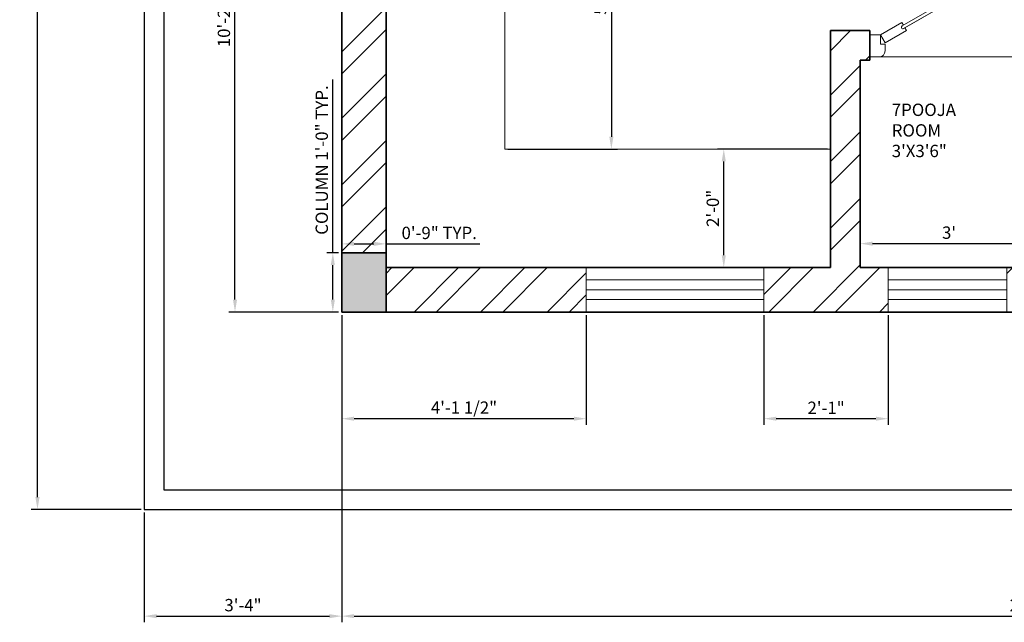
# Model space of a CAD drawing. Units: inches. Extents: x -138 to 270, y 8284 to 8764.
# Tile 1 of 10: x -138 to 61, y 8284 to 8406. Entities that reach past the tile are written whole.
import ezdxf

# ---------------------------------------------------------------- set-up
doc = ezdxf.new("R2010")
doc.units = ezdxf.units.IN
for name, color, linetype, lineweight in [('A-ANNO-DIMS', 2, 'Continuous', 18), ('A-AREA-IDEN', 7, 'Continuous', 18), ('A-FLOR-CASE', 9, 'Continuous', 18), ('C-PROP', 7, 'Continuous', 25), ('DOOR', 32, 'Continuous', 15), ('WALL', 8, 'Continuous', 35), ('WINDOW', 151, 'Continuous', 15)]:
    doc.layers.add(name, color=color, linetype=linetype, lineweight=lineweight)
doc.layers.add('A-COLS', color=252, linetype='Continuous', lineweight=35, true_color=0x939598)
doc.layers.add('A-WALL-PATT', color=32, linetype='Continuous', lineweight=9, true_color=0xbc761a)
doc.styles.get("Standard").update_dxf_attribs({"font": 'arial.ttf'})
doc.dimstyles.new('ISO-25', dxfattribs={"dimtxt": 2.5, "dimasz": 2.5, "dimexe": 1.25, "dimexo": 0.625, "dimtad": 1, "dimdec": 0, "dimlunit": 3, "dimtxsty": 'Standard', "dimcen": 2.5, "dimadec": 0, "dimazin": 0, "dimtfac": 1, "dimtdec": 0, "dimtmove": 0, "dimatfit": 3, "dimfxl": 1, "dimarcsym": 0})

# ---------------------------------------------------------------- blocks, each defined once
blk = doc.blocks.new('A$C1A8229D7')
at = {"layer": 'DOOR'}
for p, q in [((22.38, 16.16), (26.71, 18.66)), ((24.39, 17.68), (25.47, 18.3)), ((24.56, 18), (25.1, 18.31)), ((24.56, 18), (24.66, 17.83)), ((24.56, 18), (24.56, 18)), ((24.83, 18.15), (24.83, 18.15)), ((25.1, 18.31), (25.2, 18.15)), ((25.47, 18.3), (25.62, 18.03)), ((27.64, 17.03), (26.71, 18.66)), ((22.69, 15.61), (22.38, 16.16)), ((23.31, 14.53), (27.64, 17.03)), ((24.39, 17.68), (24.54, 17.41)), ((25.64, 15.51), (26.72, 16.14)), ((26.54, 15.82), (26.45, 15.98)), ((26.72, 16.14), (26.56, 16.41)), ((6.56, 6.3), (22.96, 15.77)), ((23.27, 15.23), (6.87, 5.76)), ((7.14, 5.92), (23, 15.07)), ((23.31, 14.53), (23, 15.07)), ((23.39, 15.66), (23.39, 15.66)), ((25.64, 15.51), (25.48, 15.78)), ((26, 15.51), (25.91, 15.67)), ((26, 15.51), (26.54, 15.82)), ((26, 15.51), (26, 15.51)), ((26.27, 15.66), (26.27, 15.66)), ((6.52, 7), (2.19, 4.5)), ((6.83, 6.46), (6.52, 7)), ((0, 0), (0, 4.5)), ((0, 4.5), (2.19, 4.5)), ((2.19, 2.62), (2.19, 4.5)), ((3.12, 2.88), (2.19, 4.5)), ((7.46, 5.38), (3.12, 2.88)), ((6.45, 5.88), (6.45, 5.88)), ((7.46, 5.38), (7.14, 5.92)), ((30.5, 2.62), (30.5, 4.5)), ((33, 4.5), (30.5, 4.5)), ((33, 0), (33, 4.5)), ((2.19, 2.62), (3.12, 2.62)), ((3.12, 1.25), (3.12, 2.62)), ((29.87, 1.25), (29.87, 2.62)), ((30.5, 2.62), (29.87, 2.62)), ((0, 0), (1.87, 0)), ((33, 0), (0, 0)), ((0, 0), (33, 0)), ((33, 0), (31.12, 0))]:
    blk.add_line(p, q, dxfattribs=at)
at = {"layer": 'DOOR', "ltscale": 0.1}
blk.add_arc((6.98, 5.45), 23.69, 353.1504, 56.0415, dxfattribs=at)
at = {"layer": 'DOOR'}
for centre, radius, start, end in [((25.46, 15.13), 3.63, 111.4546, 145.7774), ((27.78, 10.32), 8.61, 114.2033, 127.709), ((24.4, 17.99), 0.592, 22.7059, 117.5689), ((24.41, 17.91), 0.312, 30, 120), ((22.48, 17.15), 0.0372, 138.2373, 332.5518), ((23.12, 15.5), 0.312, 30, 120), ((23.12, 15.5), 0.312, 300, 30), ((24.23, 14.13), 0.0372, 87.4482, 281.7627), ((20.96, 22.13), 8.61, 292.291, 305.7967), ((23.97, 17.71), 3.63, 274.2226, 308.5454), ((25.85, 15.42), 0.312, 300, 30), ((25.92, 15.37), 0.592, 302.4311, 37.2941), ((6.72, 6.03), 0.312, 120, 210), ((6.72, 6.03), 0.312, 210, 300), ((1.87, 1.25), 1.25, 270, 0), ((31.12, 1.25), 1.25, 180, 270)]:
    blk.add_arc(centre, radius, start, end, dxfattribs=at)
blk = doc.blocks.new('*D24')
at = {"layer": 'A-ANNO-DIMS', "color": 0, "lineweight": -2, "transparency": 16777216}
for p, q in [((32.08, 8356.87), (32.08, 8362.34)), ((68.08, 8356.87), (68.08, 8362.34)), ((34.58, 8361.09), (65.58, 8361.09))]:
    blk.add_line(p, q, dxfattribs=at)
at = {"layer": 'A-ANNO-DIMS', "color": 0, "transparency": 16777216}
for points in [[(34.58, 8361.51), (34.58, 8360.67), (32.08, 8361.09)], [(65.58, 8361.51), (65.58, 8360.67), (68.08, 8361.09)]]:
    blk.add_solid(points, dxfattribs=at)
at = {"layer": 'Defpoints', "color": 0, "transparency": 16777216}
for p in [(68.08, 8361.09), (32.08, 8356.24), (68.08, 8356.24)]:
    blk.add_point(p, dxfattribs=at)
at = {"layer": 'A-ANNO-DIMS', "color": 0, "transparency": 16777216, "insert": (50.08, 8362.99), "char_height": 2.5, "attachment_point": 5}
blk.add_mtext("3'", dxfattribs=at)
blk = doc.blocks.new('WINDOW-36IN')
for p, q in [((0, 6.5), (36, 6.5)), ((0, 4.5), (36, 4.5)), ((0, 2.5), (36, 2.5))]:
    blk.add_line(p, q)
blk.add_lwpolyline([(0, 0), (36, 0), (36, 9), (0, 9)], close=True)
blk = doc.blocks.new('WINDOW-24IN')
for p, q in [((0, 6.5), (24, 6.5)), ((0, 4.5), (24, 4.5)), ((0, 2.5), (24, 2.5))]:
    blk.add_line(p, q)
blk.add_lwpolyline([(0, 0), (24, 0), (24, 9), (0, 9)], close=True)
blk = doc.blocks.new('COLUMN-9X12IN')
h = blk.add_hatch(color=256)
h.dxf.hatch_style = 1
h.paths.add_polyline_path([(9, 12), (0, 12), (0, 0), (9, 0)])
blk.add_lwpolyline([(0, 0), (9, 0), (9, 12), (0, 12)], close=True)
blk = doc.blocks.new('*D29')
at = {"layer": 'A-ANNO-DIMS', "color": 0, "lineweight": -2, "transparency": 16777216}
for p, q in [((-74.72, 8359.24), (-74.72, 8394.31)), ((-73.55, 8359.24), (-75.97, 8359.24)), ((-74.72, 8349.74), (-74.72, 8356.74)), ((-73.55, 8347.24), (-75.97, 8347.24))]:
    blk.add_line(p, q, dxfattribs=at)
at = {"layer": 'A-ANNO-DIMS', "color": 0, "transparency": 16777216}
for points in [[(-75.14, 8356.74), (-74.31, 8356.74), (-74.72, 8359.24)], [(-75.14, 8349.74), (-74.31, 8349.74), (-74.72, 8347.24)]]:
    blk.add_solid(points, dxfattribs=at)
at = {"layer": 'Defpoints', "color": 0, "transparency": 16777216}
for p in [(-74.72, 8359.24), (-72.92, 8359.24), (-72.92, 8347.24)]:
    blk.add_point(p, dxfattribs=at)
at = {"layer": 'A-ANNO-DIMS', "color": 0, "transparency": 16777216, "insert": (-76.64, 8378.02), "char_height": 2.5, "attachment_point": 5, "rotation": 90}
blk.add_mtext('COLUMN 1\'-0" TYP.', dxfattribs=at)
blk = doc.blocks.new('*D30')
at = {"layer": 'A-ANNO-DIMS', "color": 0, "lineweight": -2, "transparency": 16777216}
for p, q in [((-72.92, 8359.87), (-72.92, 8362.29)), ((-63.92, 8359.87), (-63.92, 8362.29)), ((-70.42, 8361.04), (-66.42, 8361.04)), ((-63.92, 8361.04), (-44.94, 8361.04))]:
    blk.add_line(p, q, dxfattribs=at)
at = {"layer": 'A-ANNO-DIMS', "color": 0, "transparency": 16777216}
for points in [[(-70.42, 8361.46), (-70.42, 8360.63), (-72.92, 8361.04)], [(-66.42, 8361.46), (-66.42, 8360.63), (-63.92, 8361.04)]]:
    blk.add_solid(points, dxfattribs=at)
at = {"layer": 'Defpoints', "color": 0, "transparency": 16777216}
for p in [(-63.92, 8361.04), (-72.92, 8359.24), (-63.92, 8359.24)]:
    blk.add_point(p, dxfattribs=at)
at = {"layer": 'A-ANNO-DIMS', "color": 0, "transparency": 16777216, "insert": (-53.18, 8362.94), "char_height": 2.5, "attachment_point": 5}
blk.add_mtext('0\'-9" TYP.', dxfattribs=at)
blk = doc.blocks.new('*D52')
at = {"layer": 'A-ANNO-DIMS', "color": 0, "lineweight": -2, "transparency": 16777216}
for p, q in [((-113.55, 8739.24), (-135.79, 8739.24)), ((-134.54, 8309.74), (-134.54, 8736.74)), ((-113.55, 8307.24), (-135.79, 8307.24))]:
    blk.add_line(p, q, dxfattribs=at)
at = {"layer": 'A-ANNO-DIMS', "color": 0, "transparency": 16777216}
for points in [[(-134.96, 8736.74), (-134.12, 8736.74), (-134.54, 8739.24)], [(-134.96, 8309.74), (-134.12, 8309.74), (-134.54, 8307.24)]]:
    blk.add_solid(points, dxfattribs=at)
at = {"layer": 'Defpoints', "color": 0, "transparency": 16777216}
for p in [(-134.54, 8739.24), (-112.92, 8739.24), (-112.92, 8307.24)]:
    blk.add_point(p, dxfattribs=at)
at = {"layer": 'A-ANNO-DIMS', "color": 0, "transparency": 16777216, "insert": (-136.44, 8523.24), "char_height": 2.5, "attachment_point": 5, "rotation": 90}
blk.add_mtext('36\'-0"', dxfattribs=at)
blk = doc.blocks.new('*D53')
at = {"layer": 'A-ANNO-DIMS', "color": 0, "lineweight": -2, "transparency": 16777216}
for p, q in [((-72.92, 8346.62), (-72.92, 8284.38)), ((207.08, 8346.62), (207.08, 8284.38)), ((-70.42, 8285.63), (204.58, 8285.63))]:
    blk.add_line(p, q, dxfattribs=at)
at = {"layer": 'A-ANNO-DIMS', "color": 0, "transparency": 16777216}
for points in [[(-70.42, 8286.04), (-70.42, 8285.21), (-72.92, 8285.63)], [(204.58, 8286.04), (204.58, 8285.21), (207.08, 8285.63)]]:
    blk.add_solid(points, dxfattribs=at)
at = {"layer": 'Defpoints', "color": 0, "transparency": 16777216}
for p in [(-72.92, 8347.24), (207.08, 8347.24), (207.08, 8285.63)]:
    blk.add_point(p, dxfattribs=at)
at = {"layer": 'A-ANNO-DIMS', "color": 0, "transparency": 16777216, "insert": (67.08, 8287.53), "char_height": 2.5, "attachment_point": 5}
blk.add_mtext('23\'-4"', dxfattribs=at)
blk = doc.blocks.new('*D55')
at = {"layer": 'A-ANNO-DIMS', "color": 0, "lineweight": -2, "transparency": 16777216}
for p, q in [((-72.92, 8346.62), (-72.92, 8284.38)), ((-112.92, 8306.62), (-112.92, 8284.38)), ((-110.42, 8285.63), (-75.42, 8285.63))]:
    blk.add_line(p, q, dxfattribs=at)
at = {"layer": 'A-ANNO-DIMS', "color": 0, "transparency": 16777216}
for points in [[(-110.42, 8286.04), (-110.42, 8285.21), (-112.92, 8285.63)], [(-75.42, 8286.04), (-75.42, 8285.21), (-72.92, 8285.63)]]:
    blk.add_solid(points, dxfattribs=at)
at = {"layer": 'Defpoints', "color": 0, "transparency": 16777216}
for p in [(-72.92, 8347.24), (-112.92, 8307.24), (-72.92, 8285.63)]:
    blk.add_point(p, dxfattribs=at)
at = {"layer": 'A-ANNO-DIMS', "color": 0, "transparency": 16777216, "insert": (-92.92, 8287.53), "char_height": 2.5, "attachment_point": 5}
blk.add_mtext('3\'-4"', dxfattribs=at)
blk = doc.blocks.new('*D58')
at = {"layer": 'A-ANNO-DIMS', "color": 0, "lineweight": -2, "transparency": 16777216}
for p, q in [((-72.92, 8346.62), (-72.92, 8324.38)), ((-23.4, 8346.62), (-23.4, 8324.38)), ((-25.9, 8325.63), (-70.42, 8325.63))]:
    blk.add_line(p, q, dxfattribs=at)
at = {"layer": 'A-ANNO-DIMS', "color": 0, "transparency": 16777216}
for points in [[(-70.42, 8326.04), (-70.42, 8325.21), (-72.92, 8325.63)], [(-25.9, 8326.04), (-25.9, 8325.21), (-23.4, 8325.63)]]:
    blk.add_solid(points, dxfattribs=at)
at = {"layer": 'Defpoints', "color": 0, "transparency": 16777216}
for p in [(-72.92, 8347.24), (-23.4, 8347.24), (-72.92, 8325.63)]:
    blk.add_point(p, dxfattribs=at)
at = {"layer": 'A-ANNO-DIMS', "color": 0, "transparency": 16777216, "insert": (-48.16, 8327.55), "char_height": 2.5, "attachment_point": 5}
blk.add_mtext('4\'-1 1/2"', dxfattribs=at)
blk = doc.blocks.new('*D59')
at = {"layer": 'A-ANNO-DIMS', "color": 0, "lineweight": -2, "transparency": 16777216}
for p, q in [((12.6, 8346.62), (12.6, 8324.38)), ((37.77, 8346.62), (37.77, 8324.38)), ((35.27, 8325.63), (15.1, 8325.63))]:
    blk.add_line(p, q, dxfattribs=at)
at = {"layer": 'A-ANNO-DIMS', "color": 0, "transparency": 16777216}
for points in [[(15.1, 8326.04), (15.1, 8325.21), (12.6, 8325.63)], [(35.27, 8326.04), (35.27, 8325.21), (37.77, 8325.63)]]:
    blk.add_solid(points, dxfattribs=at)
at = {"layer": 'Defpoints', "color": 0, "transparency": 16777216}
for p in [(12.6, 8347.24), (37.77, 8347.24), (12.6, 8325.63)]:
    blk.add_point(p, dxfattribs=at)
at = {"layer": 'A-ANNO-DIMS', "color": 0, "transparency": 16777216, "insert": (25.18, 8327.51), "char_height": 2.5, "attachment_point": 5}
blk.add_mtext('2\'-1"', dxfattribs=at)
blk = doc.blocks.new('*D64')
at = {"layer": 'A-ANNO-DIMS', "color": 0, "lineweight": -2, "transparency": 16777216}
for p, q in [((-73.55, 8469.84), (-95.79, 8469.84)), ((-94.54, 8349.74), (-94.54, 8467.34)), ((-73.55, 8347.24), (-95.79, 8347.24))]:
    blk.add_line(p, q, dxfattribs=at)
at = {"layer": 'A-ANNO-DIMS', "color": 0, "transparency": 16777216}
for points in [[(-94.96, 8467.34), (-94.12, 8467.34), (-94.54, 8469.84)], [(-94.96, 8349.74), (-94.12, 8349.74), (-94.54, 8347.24)]]:
    blk.add_solid(points, dxfattribs=at)
at = {"layer": 'Defpoints', "color": 0, "transparency": 16777216}
for p in [(-94.54, 8469.84), (-72.92, 8469.84), (-72.92, 8347.24)]:
    blk.add_point(p, dxfattribs=at)
at = {"layer": 'A-ANNO-DIMS', "color": 0, "transparency": 16777216, "insert": (-96.46, 8408.54), "char_height": 2.5, "attachment_point": 5, "rotation": 90}
blk.add_mtext('10\'-2 1/2"', dxfattribs=at)
blk = doc.blocks.new('*D74')
at = {"layer": 'A-ANNO-DIMS', "color": 0, "lineweight": -2, "transparency": 16777216}
for p, q in [((-39.3, 8442.24), (-17.06, 8442.24)), ((-18.31, 8439.74), (-18.31, 8382.74)), ((-39.3, 8380.24), (-17.06, 8380.24))]:
    blk.add_line(p, q, dxfattribs=at)
at = {"layer": 'A-ANNO-DIMS', "color": 0, "transparency": 16777216}
for points in [[(-18.73, 8439.74), (-17.89, 8439.74), (-18.31, 8442.24)], [(-18.73, 8382.74), (-17.89, 8382.74), (-18.31, 8380.24)]]:
    blk.add_solid(points, dxfattribs=at)
at = {"layer": 'Defpoints', "color": 0, "transparency": 16777216}
for p in [(-39.92, 8442.24), (-39.92, 8380.24), (-18.31, 8380.24)]:
    blk.add_point(p, dxfattribs=at)
at = {"layer": 'A-ANNO-DIMS', "color": 0, "transparency": 16777216, "insert": (-20.21, 8411.24), "char_height": 2.5, "attachment_point": 5, "rotation": 90}
blk.add_mtext('5\'-2"', dxfattribs=at)
blk = doc.blocks.new('*D75')
at = {"layer": 'A-ANNO-DIMS', "color": 0, "lineweight": -2, "transparency": 16777216}
for p, q in [((25.45, 8380.24), (3.21, 8380.24)), ((4.46, 8358.74), (4.46, 8377.74)), ((25.45, 8356.24), (3.21, 8356.24))]:
    blk.add_line(p, q, dxfattribs=at)
at = {"layer": 'A-ANNO-DIMS', "color": 0, "transparency": 16777216}
for points in [[(4.04, 8377.74), (4.88, 8377.74), (4.46, 8380.24)], [(4.04, 8358.74), (4.88, 8358.74), (4.46, 8356.24)]]:
    blk.add_solid(points, dxfattribs=at)
at = {"layer": 'Defpoints', "color": 0, "transparency": 16777216}
for p in [(4.46, 8380.24), (26.08, 8380.24), (26.08, 8356.24)]:
    blk.add_point(p, dxfattribs=at)
at = {"layer": 'A-ANNO-DIMS', "color": 0, "transparency": 16777216, "insert": (2.56, 8368.24), "char_height": 2.5, "attachment_point": 5, "rotation": 90}
blk.add_mtext('2\'-0"', dxfattribs=at)

msp = doc.modelspace()

# ---------------------------------------------------------------- hatches: boundary and pattern name
at = {"layer": 'A-WALL-PATT'}
h = msp.add_hatch(dxfattribs=at)
h.set_pattern_fill('ANSI32', color=256)
h.paths.add_polyline_path([(-23.4, 8356.24), (-63.92, 8356.24), (-63.92, 8347.24), (-23.4, 8347.24)])
h.paths.add_polyline_path([(-63.92, 8469.84), (-72.92, 8469.84), (-72.92, 8359.24), (-63.92, 8359.24)])
h.paths.add_polyline_path([(-63.92, 8510.27), (-72.92, 8510.27), (-72.92, 8505.84), (-63.92, 8505.84)])
h.paths.add_polyline_path([(-63.92, 8527.36), (-72.92, 8527.36), (-72.92, 8522.27), (-63.92, 8522.27)])
h.paths.add_polyline_path([(26.08, 8522.24), (24.78, 8522.24), (24.78, 8522.24), (20.08, 8522.24), (20.08, 8516.24), (-63.92, 8516.24), (-63.92, 8510.24), (26.08, 8510.24)])
h.paths.add_polyline_path([(34.02, 8398.24), (34.02, 8404.24), (26.08, 8404.24), (26.08, 8356.24), (12.6, 8356.24), (12.6, 8347.24), (37.77, 8347.24), (37.77, 8356.24), (32.08, 8356.24), (32.08, 8398.24)])
h.paths.add_polyline_path([(67.02, 8404.24), (67.02, 8398.24), (68.08, 8398.24), (68.08, 8356.24), (61.77, 8356.24), (61.77, 8347.24), (74.08, 8347.24), (74.08, 8356.24), (74.08, 8356.24), (74.08, 8449.75), (68.08, 8449.75), (68.08, 8404.24)])

# ---------------------------------------------------------------- linework, layer by layer
at = {"layer": 'A-FLOR-CASE'}
for p, q in [((-39.92, 8442.24), (-39.92, 8380.24)), ((-39.92, 8380.24), (26.08, 8380.24))]:
    msp.add_line(p, q, dxfattribs=at)
at = {"layer": 'C-PROP'}
for p, q in [((-112.92, 8739.24), (-112.92, 8307.24)), ((-108.92, 8735.24), (-108.92, 8311.24)), ((-108.92, 8311.24), (243.08, 8311.24)), ((-112.92, 8307.24), (247.08, 8307.24))]:
    msp.add_line(p, q, dxfattribs=at)
at = {"layer": 'WALL'}
for p, q in [((-72.92, 8528.24), (-72.92, 8347.24)), ((-63.92, 8504.24), (-63.92, 8356.24)), ((26.08, 8404.24), (26.08, 8356.24)), ((26.08, 8404.24), (34.02, 8404.24)), ((34.02, 8398.24), (34.02, 8404.24)), ((32.08, 8398.24), (32.08, 8356.24)), ((32.08, 8398.24), (34.02, 8398.24)), ((-63.92, 8356.24), (26.08, 8356.24)), ((32.08, 8356.24), (68.08, 8356.24)), ((-72.92, 8347.24), (42.08, 8347.24)), ((42.08, 8347.24), (138.08, 8347.24))]:
    msp.add_line(p, q, dxfattribs=at)

# ---------------------------------------------------------------- block references
at = {"layer": 'A-COLS'}
msp.add_blockref('COLUMN-9X12IN', (-72.92, 8347.24), dxfattribs=at)
at = {"layer": 'DOOR'}
msp.add_blockref('A$C1A8229D7', (34.02, 8398.9), dxfattribs=at)
at = {"layer": 'WINDOW'}
for name, p in [('WINDOW-36IN', (-23.4, 8347.24)), ('WINDOW-24IN', (37.77, 8347.24))]:
    msp.add_blockref(name, p, dxfattribs=at)

# ---------------------------------------------------------------- texts
at = {"layer": 'A-AREA-IDEN', "insert": (38.48, 8389.45), "char_height": 2.5, "attachment_point": 1}
msp.add_mtext_dynamic_manual_height_columns('7POOJA ROOM \\P3\'X3\'6"', width=21.6859, gutter_width=12.5, heights=[0], dxfattribs=at)

# ---------------------------------------------------------------- dimensions: what is measured, and where the dimension line sits
at = {"layer": 'A-ANNO-DIMS'}
for base, p1, p2, angle, picture, middle in [((-134.54, 8739.24), (-112.92, 8307.24), (-112.92, 8739.24), 90, '*D52', (-136.44, 8523.24)), ((-94.54, 8469.84), (-72.92, 8347.24), (-72.92, 8469.84), 90, '*D64', (-96.46, 8408.54)), ((-18.31, 8380.24), (-39.92, 8442.24), (-39.92, 8380.24), 270, '*D74', (-20.21, 8411.24)), ((4.46, 8380.24), (26.08, 8356.24), (26.08, 8380.24), 90, '*D75', (2.56, 8368.24)), ((-72.92, 8325.63), (-23.4, 8347.24), (-72.92, 8347.24), 180, '*D58', (-48.16, 8327.55)), ((12.6, 8325.63), (37.77, 8347.24), (12.6, 8347.24), 180, '*D59', (25.18, 8327.51))]:
    dim = msp.add_linear_dim(base=base, p1=p1, p2=p2, angle=angle, dimstyle='ISO-25', override={"dimdec": 1, "dimlfac": 1, "dimrnd": 0, "dimzin": 1, "dimdsep": 46, "dimlunit": 4, "dimfrac": 2}, dxfattribs=at)
    dim.commit()
    dim.dimension.update_dxf_attribs({"geometry": picture, "text_midpoint": middle})
dim = msp.add_linear_dim(base=(-74.72, 8359.24), p1=(-72.92, 8347.24), p2=(-72.92, 8359.24), angle=90, text='COLUMN <> TYP.', dimstyle='ISO-25', override={"dimdec": 1, "dimlfac": 1, "dimrnd": 0, "dimzin": 1, "dimdsep": 46, "dimlunit": 4, "dimfrac": 2}, dxfattribs=at)
dim.commit()
dim.dimension.update_dxf_attribs({"geometry": '*D29', "text_midpoint": (-76.64, 8378.02)})
dim = msp.add_linear_dim(base=(-63.92, 8361.04), p1=(-72.92, 8359.24), p2=(-63.92, 8359.24), text='<> TYP.', dimstyle='ISO-25', override={"dimdec": 1, "dimlfac": 1, "dimrnd": 0, "dimzin": 1, "dimdsep": 46, "dimlunit": 4, "dimfrac": 2}, dxfattribs=at)
dim.commit()
dim.dimension.update_dxf_attribs({"geometry": '*D30', "text_midpoint": (-53.18, 8362.94)})
dim = msp.add_aligned_dim(p1=(32.08, 8356.24), p2=(68.08, 8356.24), distance=4.85, dimstyle='ISO-25', override={"dimclrd": 0, "dimclre": 0, "dimclrt": 0}, dxfattribs=at)
dim.commit()
dim.dimension.update_dxf_attribs({"geometry": '*D24', "text_midpoint": (50.08, 8362.99)})
for base, p1, p2, picture, middle in [((-72.92, 8285.63), (-112.92, 8307.24), (-72.92, 8347.24), '*D55', (-92.92, 8287.53)), ((207.08, 8285.63), (-72.92, 8347.24), (207.08, 8347.24), '*D53', (67.08, 8287.53))]:
    dim = msp.add_linear_dim(base=base, p1=p1, p2=p2, dimstyle='ISO-25', override={"dimdec": 1, "dimlfac": 1, "dimrnd": 0, "dimzin": 1, "dimdsep": 46, "dimlunit": 4, "dimfrac": 2}, dxfattribs=at)
    dim.commit()
    dim.dimension.update_dxf_attribs({"geometry": picture, "text_midpoint": middle})

doc.saveas('drawing.dxf')
